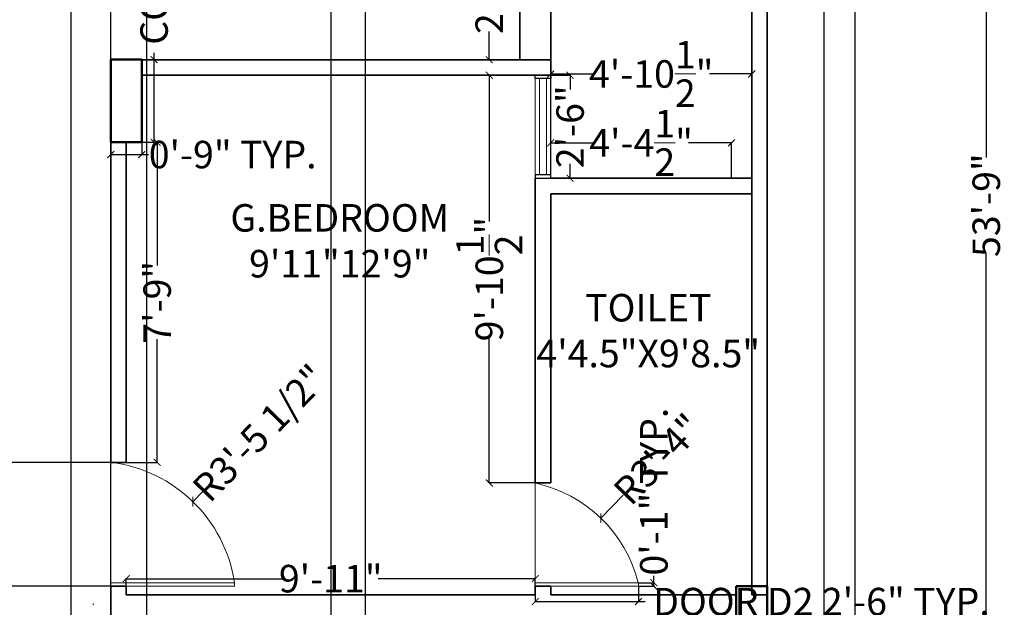
# Model space of a CAD drawing. Units: inches. Extents: x 490 to 1091, y 501 to 1322.
# Tile 3 of 5: x 804 to 1091, y 788 to 959. Entities that reach past the tile are written whole.
import ezdxf

# ---------------------------------------------------------------- set-up
doc = ezdxf.new("R2010")
doc.units = ezdxf.units.IN
doc.header["$MEASUREMENT"] = 0
for name, color, linetype, lineweight in [('A-ANNO-DIMS', 2, 'Continuous', 18), ('A-AREA-IDEN', 7, 'Continuous', 25), ('A-COLS', 12, 'Continuous', 50), ('A-DOOR', 3, 'Continuous', 20), ('A-GLAZ', 4, 'Continuous', 18), ('A-WALL', 7, 'Continuous', 35), ('C-PROP', 8, 'Continuous', 25)]:
    doc.layers.add(name, color=color, linetype=linetype, lineweight=lineweight)
doc.styles.get("Standard").update_dxf_attribs({"font": 'arial.ttf'})
doc.dimstyles.get("Standard").update_dxf_attribs({"dimtxt": 8, "dimasz": 2, "dimexe": 0.18, "dimexo": 0.0625, "dimgap": 0.09, "dimtad": 0, "dimdec": 1, "dimzin": 0, "dimdsep": 46, "dimlunit": 4, "dimtxsty": 'Standard', "dimblk": 'ARCHTICK', "dimcen": 0.09, "dimadec": 0, "dimazin": 0, "dimtfac": 1, "dimtdec": 1, "dimtofl": 0, "dimtmove": 0, "dimatfit": 3, "dimldrblk": 'ARCHTICK', "dimfxl": 1, "dimtolj": 1, "dimtzin": 0, "dimarcsym": 0})

# ---------------------------------------------------------------- blocks, each defined once
blk = doc.blocks.new('jcjg  bmvh')
for p, q in [((1232.66, 1066.6), (1223.66, 1066.6)), ((1223.66, 1066.6), (1223.66, 1042.6)), ((1232.66, 1042.6), (1232.66, 1066.6)), ((1223.66, 1042.6), (1232.66, 1042.6))]:
    blk.add_line(p, q)
blk = doc.blocks.new('bndfnhhj')
for p, q in [((1343.93, 958.21), (1348.43, 958.21)), ((1343.93, 928.21), (1343.93, 958.21)), ((1343.93, 957.21), (1348.43, 957.21)), ((1345.18, 957.21), (1345.18, 929.21)), ((1347.18, 957.21), (1347.18, 929.21)), ((1348.43, 958.21), (1348.43, 928.21)), ((1348.43, 929.21), (1343.93, 929.21)), ((1348.43, 928.21), (1343.93, 928.21))]:
    blk.add_line(p, q)
at = {"layer": 'Defpoints'}
for points in [[(1343.93, 958.21), (1348.43, 958.21), (1348.43, 957.21), (1343.93, 957.21)], [(1343.93, 928.21), (1348.43, 928.21), (1348.43, 929.21), (1343.93, 929.21)]]:
    blk.add_lwpolyline(points, close=True, dxfattribs=at)
blk = doc.blocks.new('_ArchTick')
at = {"color": 0, "linetype": 'ByBlock', "const_width": 0.15}
blk.add_lwpolyline([(-0.5, -0.5), (0.5, 0.5)], dxfattribs=at)
blk = doc.blocks.new('*D10')
at = {"layer": 'A-ANNO-DIMS', "color": 0, "lineweight": -2, "transparency": 16777216}
for p, q in [((835.17, 791.65), (835.17, 796.43)), ((954.17, 791.65), (954.17, 796.43)), ((835.17, 796.25), (880.84, 796.25)), ((954.17, 796.25), (908.5, 796.25))]:
    blk.add_line(p, q, dxfattribs=at)
at = {"layer": 'Defpoints', "color": 0, "transparency": 16777216}
for p in [(835.17, 796.25), (835.17, 791.58), (954.17, 791.58)]:
    blk.add_point(p, dxfattribs=at)
at = {"layer": 'A-ANNO-DIMS', "color": 0, "lineweight": -2, "transparency": 16777216, "xscale": 2, "yscale": 2, "zscale": 2, "rotation": 180}
blk.add_blockref('_ArchTick', (835.17, 796.25), dxfattribs=at)
at = {"layer": 'A-ANNO-DIMS', "color": 0, "lineweight": -2, "transparency": 16777216, "xscale": 2, "yscale": 2, "zscale": 2}
blk.add_blockref('_ArchTick', (954.17, 796.25), dxfattribs=at)
at = {"layer": 'A-ANNO-DIMS', "color": 0, "transparency": 16777216, "insert": (894.67, 796.25), "char_height": 8, "attachment_point": 5}
blk.add_mtext('\\A1;9\'-11"', dxfattribs=at)
blk = doc.blocks.new('*D11')
at = {"layer": 'A-ANNO-DIMS', "color": 0, "lineweight": -2, "transparency": 16777216}
for p, q in [((835.23, 923.18), (844.34, 923.18)), ((844.16, 923.18), (844.16, 887.33)), ((844.16, 830.08), (844.16, 865.94)), ((835.23, 830.08), (844.34, 830.08))]:
    blk.add_line(p, q, dxfattribs=at)
at = {"layer": 'Defpoints', "color": 0, "transparency": 16777216}
for p in [(835.17, 923.18), (844.16, 923.18), (835.17, 830.08)]:
    blk.add_point(p, dxfattribs=at)
at = {"layer": 'A-ANNO-DIMS', "color": 0, "lineweight": -2, "transparency": 16777216, "xscale": 2, "yscale": 2, "zscale": 2}
for p, rotation in [((844.16, 923.18), 90), ((844.16, 830.08), 270)]:
    blk.add_blockref('_ArchTick', p, dxfattribs=dict(at, rotation=rotation))
at = {"layer": 'A-ANNO-DIMS', "color": 0, "transparency": 16777216, "insert": (844.16, 876.63), "char_height": 8, "attachment_point": 5, "rotation": 90}
blk.add_mtext('\\A1;7\'-9"', dxfattribs=at)
blk = doc.blocks.new('*D12')
at = {"layer": 'A-ANNO-DIMS', "color": 0, "lineweight": -2, "transparency": 16777216}
for p, q in [((954.11, 942.68), (940.63, 942.68)), ((940.81, 942.68), (940.81, 900.13)), ((940.81, 824.08), (940.81, 866.64)), ((954.11, 824.08), (940.63, 824.08))]:
    blk.add_line(p, q, dxfattribs=at)
at = {"layer": 'Defpoints', "color": 0, "transparency": 16777216}
for p in [(954.17, 942.68), (940.81, 824.08), (954.17, 824.08)]:
    blk.add_point(p, dxfattribs=at)
at = {"layer": 'A-ANNO-DIMS', "color": 0, "lineweight": -2, "transparency": 16777216, "xscale": 2, "yscale": 2, "zscale": 2}
for p, rotation in [((940.81, 942.68), 90), ((940.81, 824.08), 270)]:
    blk.add_blockref('_ArchTick', p, dxfattribs=dict(at, rotation=rotation))
at = {"layer": 'A-ANNO-DIMS', "color": 0, "transparency": 16777216, "insert": (940.81, 883.38), "char_height": 8, "attachment_point": 5, "rotation": 90}
blk.add_mtext('\\A1;9\'-10{\\H1x;\\S1/2;}"', dxfattribs=at)
blk = doc.blocks.new('*D31')
at = {"layer": 'A-ANNO-DIMS', "color": 0, "lineweight": -2, "transparency": 16777216}
for p, q in [((949.61, 971.18), (940.6, 971.18)), ((940.78, 971.18), (940.78, 963.02)), ((940.78, 947.18), (940.78, 955.35)), ((949.61, 947.18), (940.6, 947.18))]:
    blk.add_line(p, q, dxfattribs=at)
at = {"layer": 'Defpoints', "color": 0, "transparency": 16777216}
for p in [(940.78, 971.18), (949.67, 971.18), (949.67, 947.18)]:
    blk.add_point(p, dxfattribs=at)
at = {"layer": 'A-ANNO-DIMS', "color": 0, "lineweight": -2, "transparency": 16777216, "xscale": 2, "yscale": 2, "zscale": 2}
for p, rotation in [((940.78, 971.18), 90), ((940.78, 947.18), 270)]:
    blk.add_blockref('_ArchTick', p, dxfattribs=dict(at, rotation=rotation))
at = {"layer": 'A-ANNO-DIMS', "color": 0, "transparency": 16777216, "insert": (940.78, 959.18), "char_height": 8, "attachment_point": 5, "rotation": 90}
blk.add_mtext("\\A1;2'", dxfattribs=at)
blk = doc.blocks.new('*D32')
at = {"layer": 'A-ANNO-DIMS', "color": 0, "lineweight": -2, "transparency": 16777216}
for p, q in [((958.73, 942.68), (964.48, 942.68)), ((964.3, 942.68), (964.3, 938.48)), ((964.3, 912.68), (964.3, 916.89)), ((958.73, 912.68), (964.48, 912.68))]:
    blk.add_line(p, q, dxfattribs=at)
at = {"layer": 'Defpoints', "color": 0, "transparency": 16777216}
for p in [(958.67, 942.68), (958.67, 912.68), (964.3, 912.68)]:
    blk.add_point(p, dxfattribs=at)
at = {"layer": 'A-ANNO-DIMS', "color": 0, "lineweight": -2, "transparency": 16777216, "xscale": 2, "yscale": 2, "zscale": 2}
for p, rotation in [((964.3, 942.68), 90), ((964.3, 912.68), 270)]:
    blk.add_blockref('_ArchTick', p, dxfattribs=dict(at, rotation=rotation))
at = {"layer": 'A-ANNO-DIMS', "color": 0, "transparency": 16777216, "insert": (964.3, 927.68), "char_height": 8, "attachment_point": 5, "rotation": 90}
blk.add_mtext('\\A1;2\'-6"', dxfattribs=at)
blk = doc.blocks.new('*D33')
at = {"layer": 'A-ANNO-DIMS', "color": 0, "lineweight": -2, "transparency": 16777216}
for p, q in [((958.67, 912.75), (958.67, 923.16)), ((958.67, 922.98), (971.17, 922.98)), ((1011.27, 922.98), (998.77, 922.98)), ((1011.27, 912.75), (1011.27, 923.16))]:
    blk.add_line(p, q, dxfattribs=at)
at = {"layer": 'Defpoints', "color": 0, "transparency": 16777216}
for p in [(1011.27, 922.98), (958.67, 912.68), (1011.27, 912.68)]:
    blk.add_point(p, dxfattribs=at)
at = {"layer": 'A-ANNO-DIMS', "color": 0, "lineweight": -2, "transparency": 16777216, "xscale": 2, "yscale": 2, "zscale": 2, "rotation": 180}
blk.add_blockref('_ArchTick', (958.67, 922.98), dxfattribs=at)
at = {"layer": 'A-ANNO-DIMS', "color": 0, "lineweight": -2, "transparency": 16777216, "xscale": 2, "yscale": 2, "zscale": 2}
blk.add_blockref('_ArchTick', (1011.27, 922.98), dxfattribs=at)
at = {"layer": 'A-ANNO-DIMS', "color": 0, "transparency": 16777216, "insert": (984.97, 922.98), "char_height": 8, "attachment_point": 5}
blk.add_mtext('\\A1;4\'-4{\\H1x;\\S1/2;}"', dxfattribs=at)
blk = doc.blocks.new('*D34')
at = {"layer": 'A-ANNO-DIMS', "color": 0, "lineweight": -2, "transparency": 16777216}
for p, q in [((958.67, 912.75), (958.67, 943.21)), ((958.67, 943.03), (971.01, 943.03)), ((1017.17, 943.03), (1004.83, 943.03)), ((1017.17, 912.75), (1017.17, 943.21))]:
    blk.add_line(p, q, dxfattribs=at)
at = {"layer": 'Defpoints', "color": 0, "transparency": 16777216}
for p in [(1017.17, 943.03), (958.67, 912.68), (1017.17, 912.68)]:
    blk.add_point(p, dxfattribs=at)
at = {"layer": 'A-ANNO-DIMS', "color": 0, "lineweight": -2, "transparency": 16777216, "xscale": 2, "yscale": 2, "zscale": 2, "rotation": 180}
blk.add_blockref('_ArchTick', (958.67, 943.03), dxfattribs=at)
at = {"layer": 'A-ANNO-DIMS', "color": 0, "lineweight": -2, "transparency": 16777216, "xscale": 2, "yscale": 2, "zscale": 2}
blk.add_blockref('_ArchTick', (1017.17, 943.03), dxfattribs=at)
at = {"layer": 'A-ANNO-DIMS', "color": 0, "transparency": 16777216, "insert": (987.92, 943.03), "char_height": 8, "attachment_point": 5}
blk.add_mtext('\\A1;4\'-10{\\H1x;\\S1/2;}"', dxfattribs=at)
blk = doc.blocks.new('DOOR-LEAF-30IN')
for p, q in [((0, 0), (0, 1)), ((0, 1), (30, 1)), ((30, 0), (0, 0)), ((30, 1), (30, 0))]:
    blk.add_line(p, q)
blk = doc.blocks.new('*D50')
at = {"layer": 'A-ANNO-DIMS', "color": 0, "lineweight": -2, "transparency": 16777216}
for p, q in [((843.27, 947.18), (843.27, 949.18)), ((839.73, 947.18), (843.45, 947.18)), ((843.27, 923.18), (843.27, 947.18)), ((839.73, 923.18), (843.45, 923.18))]:
    blk.add_line(p, q, dxfattribs=at)
at = {"layer": 'Defpoints', "color": 0, "transparency": 16777216}
for p in [(839.67, 947.18), (843.27, 947.18), (839.67, 923.18)]:
    blk.add_point(p, dxfattribs=at)
at = {"layer": 'A-ANNO-DIMS', "color": 0, "lineweight": -2, "transparency": 16777216, "xscale": 2, "yscale": 2, "zscale": 2}
for p, rotation in [((843.27, 947.18), 90), ((843.27, 923.18), 270)]:
    blk.add_blockref('_ArchTick', p, dxfattribs=dict(at, rotation=rotation))
at = {"layer": 'A-ANNO-DIMS', "color": 0, "transparency": 16777216, "insert": (843.27, 996.9), "char_height": 8, "attachment_point": 5, "rotation": 90}
blk.add_mtext('\\A1;COL. C2 2\'-0" TYP.', dxfattribs=at)
blk = doc.blocks.new('*D51')
at = {"layer": 'A-ANNO-DIMS', "color": 0, "lineweight": -2, "transparency": 16777216}
for p, q in [((830.67, 923.12), (830.67, 919.4)), ((839.67, 923.12), (839.67, 919.4)), ((830.67, 919.58), (839.67, 919.58)), ((839.67, 919.58), (841.67, 919.58))]:
    blk.add_line(p, q, dxfattribs=at)
at = {"layer": 'Defpoints', "color": 0, "transparency": 16777216}
for p in [(830.67, 923.18), (839.67, 923.18), (839.67, 919.58)]:
    blk.add_point(p, dxfattribs=at)
at = {"layer": 'A-ANNO-DIMS', "color": 0, "lineweight": -2, "transparency": 16777216, "xscale": 2, "yscale": 2, "zscale": 2, "rotation": 180}
blk.add_blockref('_ArchTick', (830.67, 919.58), dxfattribs=at)
at = {"layer": 'A-ANNO-DIMS', "color": 0, "lineweight": -2, "transparency": 16777216, "xscale": 2, "yscale": 2, "zscale": 2}
blk.add_blockref('_ArchTick', (839.67, 919.58), dxfattribs=at)
at = {"layer": 'A-ANNO-DIMS', "color": 0, "transparency": 16777216, "insert": (866.14, 919.58), "char_height": 8, "attachment_point": 5}
blk.add_mtext('\\A1;0\'-9" TYP.', dxfattribs=at)
blk = doc.blocks.new('*D56')
at = {"layer": 'A-ANNO-DIMS', "color": 0, "lineweight": -2, "transparency": 16777216}
for p, q in [((954.17, 794.02), (954.17, 789.4)), ((984.17, 794.02), (984.17, 789.4)), ((954.17, 789.58), (984.17, 789.58)), ((984.17, 789.58), (986.17, 789.58))]:
    blk.add_line(p, q, dxfattribs=at)
at = {"layer": 'Defpoints', "color": 0, "transparency": 16777216}
for p in [(954.17, 794.08), (984.17, 794.08), (984.17, 789.58)]:
    blk.add_point(p, dxfattribs=at)
at = {"layer": 'A-ANNO-DIMS', "color": 0, "lineweight": -2, "transparency": 16777216, "xscale": 2, "yscale": 2, "zscale": 2, "rotation": 180}
blk.add_blockref('_ArchTick', (954.17, 789.58), dxfattribs=at)
at = {"layer": 'A-ANNO-DIMS', "color": 0, "lineweight": -2, "transparency": 16777216, "xscale": 2, "yscale": 2, "zscale": 2}
blk.add_blockref('_ArchTick', (984.17, 789.58), dxfattribs=at)
at = {"layer": 'A-ANNO-DIMS', "color": 0, "transparency": 16777216, "insert": (1037.45, 789.58), "char_height": 8, "attachment_point": 5}
blk.add_mtext('\\A1;DOOR D2 2\'-6" TYP.', dxfattribs=at)
blk = doc.blocks.new('*D57')
at = {"layer": 'A-ANNO-DIMS', "color": 0, "lineweight": -2, "transparency": 16777216}
for p, q in [((988.67, 795.08), (988.67, 797.08)), ((984.23, 795.08), (988.85, 795.08)), ((984.23, 794.08), (988.85, 794.08)), ((988.67, 794.08), (988.67, 795.08))]:
    blk.add_line(p, q, dxfattribs=at)
at = {"layer": 'Defpoints', "color": 0, "transparency": 16777216}
for p in [(984.17, 795.08), (984.17, 794.08), (988.67, 795.08)]:
    blk.add_point(p, dxfattribs=at)
at = {"layer": 'A-ANNO-DIMS', "color": 0, "lineweight": -2, "transparency": 16777216, "xscale": 2, "yscale": 2, "zscale": 2}
for p, rotation in [((988.67, 795.08), 90), ((988.67, 794.08), 270)]:
    blk.add_blockref('_ArchTick', p, dxfattribs=dict(at, rotation=rotation))
at = {"layer": 'A-ANNO-DIMS', "color": 0, "transparency": 16777216, "insert": (988.67, 821.56), "char_height": 8, "attachment_point": 5, "rotation": 90}
blk.add_mtext('\\A1;0\'-1" TYP.', dxfattribs=at)
blk = doc.blocks.new('*D65')
at = {"layer": 'A-ANNO-DIMS', "color": 0, "lineweight": -2, "transparency": 16777216}
for p, q in [((1021.73, 1227.28), (1085.58, 1227.28)), ((1085.4, 1227.28), (1085.4, 918.72)), ((1085.4, 582.48), (1085.4, 891.05)), ((1021.73, 582.48), (1085.58, 582.48))]:
    blk.add_line(p, q, dxfattribs=at)
at = {"layer": 'Defpoints', "color": 0, "transparency": 16777216}
for p in [(1021.67, 1227.28), (1085.4, 1227.28), (1021.67, 582.48)]:
    blk.add_point(p, dxfattribs=at)
at = {"layer": 'A-ANNO-DIMS', "color": 0, "lineweight": -2, "transparency": 16777216, "xscale": 2, "yscale": 2, "zscale": 2}
for p, rotation in [((1085.4, 1227.28), 90), ((1085.4, 582.48), 270)]:
    blk.add_blockref('_ArchTick', p, dxfattribs=dict(at, rotation=rotation))
at = {"layer": 'A-ANNO-DIMS', "color": 0, "transparency": 16777216, "insert": (1085.4, 904.88), "char_height": 8, "attachment_point": 5, "rotation": 90}
blk.add_mtext('\\A1;53\'-9"', dxfattribs=at)
blk = doc.blocks.new('*D69')
at = {"layer": 'A-ANNO-DIMS', "color": 0, "lineweight": -2, "transparency": 16777216}
for p, q in [((894.67, 1182.97), (894.67, 512.57)), ((904.67, 1182.97), (904.67, 512.57)), ((894.67, 512.75), (904.67, 512.75)), ((904.67, 512.75), (906.67, 512.75))]:
    blk.add_line(p, q, dxfattribs=at)
at = {"layer": 'Defpoints', "color": 0, "transparency": 16777216}
for p in [(894.67, 1183.03), (904.67, 1183.03), (904.67, 512.75)]:
    blk.add_point(p, dxfattribs=at)
at = {"layer": 'A-ANNO-DIMS', "color": 0, "lineweight": -2, "transparency": 16777216, "xscale": 2, "yscale": 2, "zscale": 2, "rotation": 180}
blk.add_blockref('_ArchTick', (894.67, 512.75), dxfattribs=at)
at = {"layer": 'A-ANNO-DIMS', "color": 0, "lineweight": -2, "transparency": 16777216, "xscale": 2, "yscale": 2, "zscale": 2}
blk.add_blockref('_ArchTick', (904.67, 512.75), dxfattribs=at)
at = {"layer": 'A-ANNO-DIMS', "color": 0, "transparency": 16777216, "insert": (920.5, 512.75), "char_height": 8, "attachment_point": 5}
blk.add_mtext('\\A1;0\'-10"', dxfattribs=at)
blk = doc.blocks.new('*D71')
at = {"layer": 'A-ANNO-DIMS', "color": 0, "lineweight": -2, "transparency": 16777216}
for p, q in [((819.07, 1134.22), (819.07, 512.57)), ((841.07, 1134.22), (841.07, 512.57)), ((819.07, 512.75), (841.07, 512.75)), ((841.07, 512.75), (843.07, 512.75))]:
    blk.add_line(p, q, dxfattribs=at)
at = {"layer": 'Defpoints', "color": 0, "transparency": 16777216}
for p in [(819.07, 1134.28), (841.07, 1134.28), (841.07, 512.75)]:
    blk.add_point(p, dxfattribs=at)
at = {"layer": 'A-ANNO-DIMS', "color": 0, "lineweight": -2, "transparency": 16777216, "xscale": 2, "yscale": 2, "zscale": 2, "rotation": 180}
blk.add_blockref('_ArchTick', (819.07, 512.75), dxfattribs=at)
at = {"layer": 'A-ANNO-DIMS', "color": 0, "lineweight": -2, "transparency": 16777216, "xscale": 2, "yscale": 2, "zscale": 2}
blk.add_blockref('_ArchTick', (841.07, 512.75), dxfattribs=at)
at = {"layer": 'A-ANNO-DIMS', "color": 0, "transparency": 16777216, "insert": (856.52, 512.75), "char_height": 8, "attachment_point": 5}
blk.add_mtext('\\A1;1\'-10"', dxfattribs=at)
blk = doc.blocks.new('*D76')
at = {"layer": 'A-ANNO-DIMS', "color": 0, "lineweight": -2, "transparency": 16777216}
for p, q in [((748.47, 802.15), (748.47, 1309.19)), ((748.47, 1309.01), (775.72, 1309.01)), ((830.67, 1309.01), (803.42, 1309.01)), ((830.67, 794.15), (830.67, 1309.19))]:
    blk.add_line(p, q, dxfattribs=at)
at = {"layer": 'Defpoints', "color": 0, "transparency": 16777216}
for p in [(830.67, 1309.01), (748.47, 802.08), (830.67, 794.08)]:
    blk.add_point(p, dxfattribs=at)
at = {"layer": 'A-ANNO-DIMS', "color": 0, "lineweight": -2, "transparency": 16777216, "xscale": 2, "yscale": 2, "zscale": 2, "rotation": 180}
blk.add_blockref('_ArchTick', (748.47, 1309.01), dxfattribs=at)
at = {"layer": 'A-ANNO-DIMS', "color": 0, "lineweight": -2, "transparency": 16777216, "xscale": 2, "yscale": 2, "zscale": 2}
blk.add_blockref('_ArchTick', (830.67, 1309.01), dxfattribs=at)
at = {"layer": 'A-ANNO-DIMS', "color": 0, "transparency": 16777216, "insert": (789.57, 1309.01), "char_height": 8, "attachment_point": 5}
blk.add_mtext('\\A1;6\'-10"', dxfattribs=at)
blk = doc.blocks.new('*D79')
at = {"layer": 'A-ANNO-DIMS', "color": 0, "lineweight": -2, "transparency": 16777216}
for p, q in [((830.61, 830.08), (528.96, 830.08)), ((529.14, 830.08), (529.14, 822.81)), ((529.14, 794.08), (529.14, 801.36)), ((830.61, 794.08), (528.96, 794.08))]:
    blk.add_line(p, q, dxfattribs=at)
at = {"layer": 'Defpoints', "color": 0, "transparency": 16777216}
for p in [(529.14, 830.08), (830.67, 830.08), (830.67, 794.08)]:
    blk.add_point(p, dxfattribs=at)
at = {"layer": 'A-ANNO-DIMS', "color": 0, "lineweight": -2, "transparency": 16777216, "xscale": 2, "yscale": 2, "zscale": 2}
for p, rotation in [((529.14, 830.08), 90), ((529.14, 794.08), 270)]:
    blk.add_blockref('_ArchTick', p, dxfattribs=dict(at, rotation=rotation))
at = {"layer": 'A-ANNO-DIMS', "color": 0, "transparency": 16777216, "insert": (529.14, 812.08), "char_height": 8, "attachment_point": 5, "rotation": 90}
blk.add_mtext('\\A1;3\'-0"', dxfattribs=at)
blk = doc.blocks.new('*D81')
at = {"layer": 'A-ANNO-DIMS', "color": 0, "lineweight": -2, "transparency": 16777216}
for p, q in [((857.34, 821.51), (854.56, 818.64)), ((825.51, 788.85), (825.69, 788.85)), ((825.6, 788.76), (825.6, 788.94))]:
    blk.add_line(p, q, dxfattribs=at)
at = {"layer": 'Defpoints', "color": 0, "transparency": 16777216}
for p in [(854.56, 818.64), (825.6, 788.85)]:
    blk.add_point(p, dxfattribs=at)
at = {"layer": 'A-ANNO-DIMS', "color": 0, "lineweight": -2, "transparency": 16777216, "xscale": 2, "yscale": 2, "zscale": 2, "rotation": 225.8067843643886}
blk.add_blockref('_ArchTick', (854.56, 818.64), dxfattribs=at)
at = {"layer": 'A-ANNO-DIMS', "color": 0, "transparency": 16777216, "insert": (873.98, 838.62), "char_height": 8, "attachment_point": 5, "rotation": 45.8068}
blk.add_mtext('\\A1;R3\'-5 1/2"', dxfattribs=at)
blk = doc.blocks.new('*D82')
at = {"layer": 'A-ANNO-DIMS', "color": 0, "lineweight": -2, "transparency": 16777216}
for p, q in [((979.77, 820.56), (973.27, 813.82)), ((945.48, 785.17), (945.66, 785.17)), ((945.57, 785.08), (945.57, 785.26))]:
    blk.add_line(p, q, dxfattribs=at)
at = {"layer": 'Defpoints', "color": 0, "transparency": 16777216}
for p in [(973.27, 813.82), (945.57, 785.17)]:
    blk.add_point(p, dxfattribs=at)
at = {"layer": 'A-ANNO-DIMS', "color": 0, "lineweight": -2, "transparency": 16777216, "xscale": 2, "yscale": 2, "zscale": 2, "rotation": 225.9717309641953}
blk.add_blockref('_ArchTick', (973.27, 813.82), dxfattribs=at)
at = {"layer": 'A-ANNO-DIMS', "color": 0, "transparency": 16777216, "insert": (989.89, 831.02), "char_height": 8, "attachment_point": 5, "rotation": 45.9717}
blk.add_mtext('\\A1;R3\'-4"', dxfattribs=at)

msp = doc.modelspace()

# ---------------------------------------------------------------- linework, layer by layer
at = {"layer": 'A-DOOR'}
for p, q in [((830.67, 794.08), (830.67, 830.08)), ((954.17, 795.08), (954.17, 824.08)), ((866.67, 795.08), (830.67, 795.08)), ((830.67, 795.08), (830.67, 794.08)), ((830.67, 794.08), (866.67, 794.08)), ((866.67, 794.08), (866.67, 795.08))]:
    msp.add_line(p, q, dxfattribs=at)
for centre, radius, start, end in [((825.6, 788.85), 41.54, 8.6276, 82.9863), ((945.57, 785.17), 39.85, 14.4043, 77.5378)]:
    msp.add_arc(centre, radius, start, end, dxfattribs=at)
at = {"layer": 'A-WALL'}
for p, q in [((1021.67, 791.58), (1021.67, 1227.28)), ((1017.17, 1049.78), (1017.17, 791.58)), ((949.67, 947.18), (949.67, 971.18)), ((958.67, 971.18), (958.67, 947.18)), ((949.67, 947.18), (830.67, 947.18)), ((830.67, 830.08), (830.67, 947.18)), ((838.07, 947.18), (835.17, 947.18)), ((958.67, 947.18), (949.67, 947.18)), ((958.67, 947.18), (958.67, 942.68)), ((839.67, 942.68), (949.67, 942.68)), ((954.17, 942.68), (949.67, 942.68)), ((958.67, 942.68), (954.17, 942.68)), ((835.17, 830.08), (835.17, 923.18)), ((954.17, 824.08), (954.17, 912.68)), ((958.67, 912.68), (1011.27, 912.68)), ((1011.27, 912.68), (1017.17, 912.68)), ((958.67, 908.18), (1011.27, 908.18)), ((958.67, 908.18), (958.67, 824.08)), ((1011.27, 908.18), (1017.17, 908.18)), ((835.17, 830.08), (830.67, 830.08)), ((954.17, 824.08), (958.67, 824.08)), ((835.17, 794.08), (830.67, 794.08)), ((830.67, 731.83), (830.67, 794.08)), ((835.17, 791.58), (835.17, 794.08)), ((835.17, 791.58), (835.17, 794.08)), ((954.17, 791.58), (954.17, 794.08)), ((958.67, 794.08), (954.17, 794.08)), ((958.67, 794.08), (958.67, 791.58)), ((954.17, 791.58), (835.17, 791.58)), ((958.67, 791.58), (1012.67, 791.58)), ((1017.17, 791.58), (1021.67, 791.58))]:
    msp.add_line(p, q, dxfattribs=at)
at = {"layer": 'C-PROP'}
for p, q in [((1047.27, 550.88), (1047.27, 1270.88)), ((1038.27, 559.88), (1038.27, 1261.88))]:
    msp.add_line(p, q, dxfattribs=at)

# ---------------------------------------------------------------- block references
at = {"layer": 'A-COLS'}
for p in [(-392.99, -119.41), (-210.99, -272.51)]:
    msp.add_blockref('jcjg  bmvh', p, dxfattribs=at)
at = {"layer": 'A-DOOR'}
msp.add_blockref('DOOR-LEAF-30IN', (954.17, 794.08), dxfattribs=at)
at = {"layer": 'A-GLAZ'}
msp.add_blockref('bndfnhhj', (-389.76, -15.52), dxfattribs=at)

# ---------------------------------------------------------------- texts
at = {"layer": 'A-AREA-IDEN', "char_height": 8, "attachment_point": 1}
for s, width, insert in [('\\pxqc;G.BEDROOM\\P9\'11"12\'9"', 58.2457, (868.17, 905.18)), ('\\pxqc;TOILET\\P4\'4.5"X9\'8.5"', 50.6284, (961.74, 879.05))]:
    msp.add_mtext_dynamic_manual_height_columns(s, width=width, gutter_width=40, heights=[0], dxfattribs=dict(at, insert=insert))

# ---------------------------------------------------------------- dimensions: what is measured, and where the dimension line sits
at = {"layer": 'A-ANNO-DIMS'}
for base, p1, p2, override, picture, middle in [((830.67, 1309.01), (748.47, 802.08), (830.67, 794.08), {"dimdec": 1, "dimlfac": 1, "dimrnd": 0, "dimzin": 1, "dimdsep": 46, "dimlunit": 4, "dimfrac": 2}, '*D76', (789.57, 1309.01)), ((904.67, 512.75), (894.67, 1183.03), (904.67, 1183.03), {"dimdec": 1, "dimlfac": 1, "dimrnd": 0, "dimzin": 1, "dimdsep": 46, "dimlunit": 4, "dimfrac": 2}, '*D69', (920.5, 512.75)), ((841.07, 512.75), (819.07, 1134.28), (841.07, 1134.28), {"dimdec": 1, "dimlfac": 1, "dimrnd": 0, "dimzin": 1, "dimdsep": 46, "dimlunit": 4, "dimfrac": 2}, '*D71', (856.52, 512.75)), ((1017.17, 943.03), (958.67, 912.68), (1017.17, 912.68), {"dimclrd": 0, "dimclre": 0, "dimclrt": 0}, '*D34', (987.92, 943.03)), ((1011.27, 922.98), (958.67, 912.68), (1011.27, 912.68), {"dimclrd": 0, "dimclre": 0, "dimclrt": 0}, '*D33', (984.97, 922.98)), ((835.17, 796.25), (954.17, 791.58), (835.17, 791.58), {"dimclrd": 0, "dimclre": 0, "dimclrt": 0}, '*D10', (894.67, 796.25))]:
    dim = msp.add_linear_dim(base=base, p1=p1, p2=p2, dimstyle='Standard', override=override, dxfattribs=at)
    dim.commit()
    dim.dimension.update_dxf_attribs({"geometry": picture, "text_midpoint": middle})
for base, p1, p2, override, picture, middle in [((1085.4, 1227.28), (1021.67, 582.48), (1021.67, 1227.28), {"dimdec": 1, "dimlfac": 1, "dimrnd": 0, "dimzin": 1, "dimdsep": 46, "dimlunit": 4, "dimfrac": 2}, '*D65', (1085.4, 904.88)), ((940.78, 971.18), (949.67, 947.18), (949.67, 971.18), {"dimclrd": 0, "dimclre": 0, "dimclrt": 0}, '*D31', (940.78, 959.18)), ((940.81, 824.08), (954.17, 942.68), (954.17, 824.08), {"dimclrd": 0, "dimclre": 0, "dimclrt": 0}, '*D12', (940.81, 883.38)), ((964.3, 912.68), (958.67, 942.68), (958.67, 912.68), {"dimclrd": 0, "dimclre": 0, "dimclrt": 0}, '*D32', (964.3, 927.68)), ((844.16, 923.18), (835.17, 830.08), (835.17, 923.18), {"dimclrd": 0, "dimclre": 0, "dimclrt": 0}, '*D11', (844.16, 876.63)), ((529.14, 830.08), (830.67, 794.08), (830.67, 830.08), {"dimdec": 1, "dimlfac": 1, "dimrnd": 0, "dimzin": 1, "dimdsep": 46, "dimlunit": 4, "dimfrac": 2}, '*D79', (529.14, 812.08))]:
    dim = msp.add_linear_dim(base=base, p1=p1, p2=p2, angle=90, dimstyle='Standard', override=override, dxfattribs=at)
    dim.commit()
    dim.dimension.update_dxf_attribs({"geometry": picture, "text_midpoint": middle})
for base, p1, p2, text, picture, middle in [((843.27, 947.18), (839.67, 923.18), (839.67, 947.18), 'COL. C2 <> TYP.', '*D50', (843.27, 996.9)), ((988.67, 795.08), (984.17, 794.08), (984.17, 795.08), '<> TYP.', '*D57', (988.67, 821.56))]:
    dim = msp.add_linear_dim(base=base, p1=p1, p2=p2, angle=90, text=text, dimstyle='Standard', override={"dimdec": 1, "dimlfac": 1, "dimrnd": 0, "dimzin": 1, "dimdsep": 46, "dimlunit": 4, "dimfrac": 2}, dxfattribs=at)
    dim.commit()
    dim.dimension.update_dxf_attribs({"geometry": picture, "text_midpoint": middle})
for base, p1, p2, text, picture, middle in [((839.67, 919.58), (830.67, 923.18), (839.67, 923.18), '<> TYP.', '*D51', (866.14, 919.58)), ((984.17, 789.58), (954.17, 794.08), (984.17, 794.08), 'DOOR D2 <> TYP.', '*D56', (1037.45, 789.58))]:
    dim = msp.add_linear_dim(base=base, p1=p1, p2=p2, text=text, dimstyle='Standard', override={"dimdec": 1, "dimlfac": 1, "dimrnd": 0, "dimzin": 1, "dimdsep": 46, "dimlunit": 4, "dimfrac": 2}, dxfattribs=at)
    dim.commit()
    dim.dimension.update_dxf_attribs({"geometry": picture, "text_midpoint": middle})
dim = msp.add_radius_dim(center=(825.6, 788.85), mpoint=(854.56, 818.64), dimstyle='Standard', override={"dimdec": 1, "dimlfac": 1, "dimrnd": 0, "dimzin": 1, "dimdsep": 46, "dimlunit": 4, "dimfrac": 2}, dxfattribs=at)
dim.commit()
dim.dimension.update_dxf_attribs({"geometry": '*D81', "text_midpoint": (873.98, 838.62)})
dim = msp.add_radius_dim(center=(945.57, 785.17), mpoint=(973.27, 813.82), dimstyle='Standard', override={"dimdec": 1, "dimlfac": 1, "dimrnd": 0, "dimzin": 1, "dimdsep": 46, "dimlunit": 4, "dimfrac": 2}, dxfattribs=at)
dim.commit()
dim.dimension.update_dxf_attribs({"geometry": '*D82', "text_midpoint": (989.89, 831.02), "dimtype": 164})

doc.saveas('drawing.dxf')
